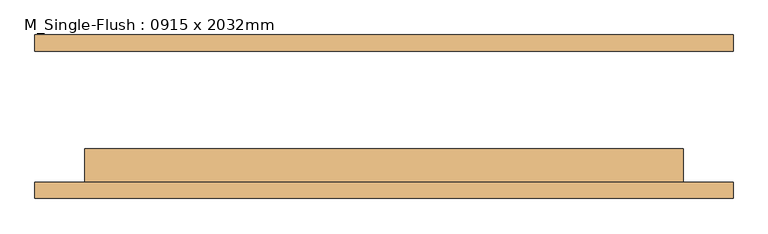
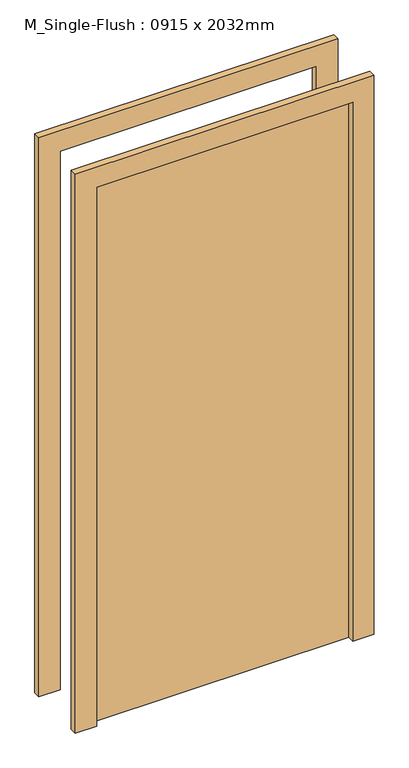
"""IFC4 building model written with IfcOpenShell, lengths in millimetres: door geometry, M_Single-Flush : 0915 x 2032mm."""

from ifc_helpers import new_model, si_unit, frame, origin, origin_with_axes, place, context, project, spatial, polyline, outline, extrude, source, transform, mapped, element, save


def m_single_flush_0915_x_2032mm_26613924(model_context):
    return source(origin(), model_context, "Body", "SweptSolid", [
        extrude(outline(polyline([(2108.0, -533.5), (0.0, -533.5), (0.0, -457.5), (2032.0, -457.5), (2032.0, 457.5), (0.0, 457.5), (0.0, 533.5), (2108.0, 533.5), (2108.0, -533.5)])), frame((0.0, -125.0, 0.0), z_axis=(0.0, 1.0, 0.0), x_axis=(0.0, 0.0, 1.0)), (0.0, 0.0, 1.0), 25.0),
        extrude(outline(polyline([(2108.0, 533.5), (2108.0, -533.5), (0.0, -533.5), (0.0, -457.5), (2032.0, -457.5), (2032.0, 457.5), (0.0, 457.5), (0.0, 533.5), (2108.0, 533.5)])), frame((0.0, 100.0, 0.0), z_axis=(0.0, 1.0, 0.0), x_axis=(0.0, 0.0, 1.0)), (0.0, 0.0, 1.0), 25.0),
        extrude(outline(polyline([(457.5, -49.0), (457.5, -100.0), (-457.5, -100.0), (-457.5, -49.0), (457.5, -49.0)])), origin_with_axes(), (0.0, 0.0, 1.0), 2032.0),
    ])


if __name__ == "__main__":
    model = new_model("IFC4")
    model_context = context("Model", 3, world=origin())
    ifc_project = project(units=[si_unit("LENGTHUNIT", "METRE", prefix="MILLI")], contexts=[model_context])
    site = spatial("IfcSite", under=ifc_project)
    building = spatial("IfcBuilding", under=site)
    placement = place(None, origin())
    m_single_flush_0915_x_2032mm_shape = m_single_flush_0915_x_2032mm_26613924(model_context)
    element("IfcDoor", 1, ObjectType="M_Single-Flush : 0915 x 2032mm", at=placement, inside=building, context=model_context, shape_type="MappedRepresentation", body=[
        mapped(m_single_flush_0915_x_2032mm_shape, transform((0.0, 0.0, 0.0), x_axis=(1.0, 0.0, 0.0), y_axis=(0.0, 1.0, 0.0), z_axis=(0.0, 0.0, 1.0))),
    ])
    save(model, "model.ifc")

# Revit data of these elements
# Type "M_Single-Flush : 0915 x 2032mm"
#   Type Mark = "20"
#   Thickness = 51 mm
#   Height = 2032 mm
#   Trim Projection Ext = 25 mm
#   Trim Projection Int = 25 mm
#   Trim Width = 76 mm
#   Width = 915 mm
#   Door Material = Door - Panel
#   Frame Material = Door - Frame
#   Function = (empty or 0)
#   Wall Closure = (empty or 0)
# Element 1 (IfcDoor, "M_Single-Flush : 0915 x 2032mm")
#   Materials on its faces: "Door - Frame", "Door - Panel"
# Materials
#   "Door - Panel": class "Wood", colour RGB 114 82 51, transparency 0
#   "Door - Frame": colour RGB 153 76 43, transparency 0
